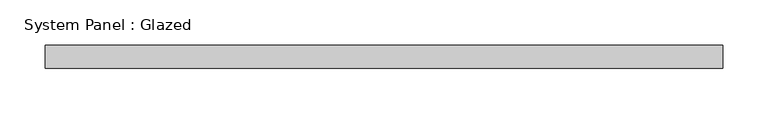
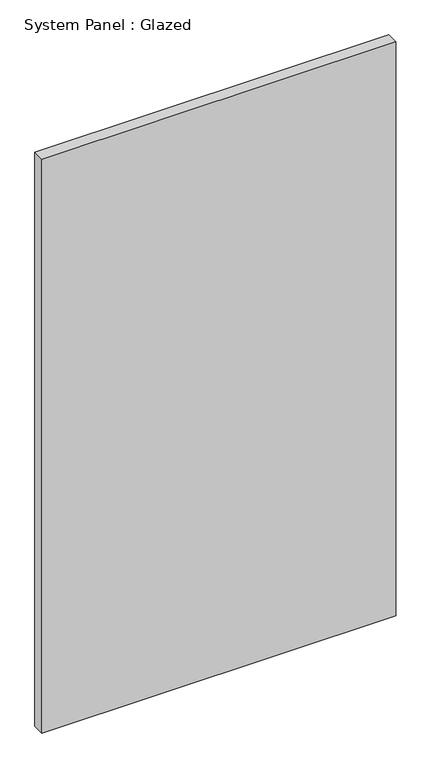
"""IFC4 building model written with IfcOpenShell, lengths in millimetres: plate geometry, System Panel : Glazed."""

from ifc_helpers import new_model, si_unit, origin, origin_with_axes, place, context, project, spatial, polyline, outline, extrude, source, transform, mapped, element, save


def system_panel_glazed_5516fd1f(model_context):
    return source(origin(), model_context, "Body", "SweptSolid", [
        extrude(outline(polyline([(374.65, 19.05), (-374.65, 19.05), (-374.65, 44.45), (374.65, 44.45), (374.65, 19.05)])), origin_with_axes(), (0.0, 0.0, 1.0), 1284.7908292),
    ])


if __name__ == "__main__":
    model = new_model("IFC4")
    model_context = context("Model", 3, world=origin())
    ifc_project = project(units=[si_unit("LENGTHUNIT", "METRE", prefix="MILLI")], contexts=[model_context])
    site = spatial("IfcSite", under=ifc_project)
    building = spatial("IfcBuilding", under=site)
    placement = place(None, origin())
    system_panel_glazed_shape = system_panel_glazed_5516fd1f(model_context)
    element("IfcPlate", 1, ObjectType="System Panel : Glazed", at=placement, inside=building, context=model_context, shape_type="MappedRepresentation", body=[
        mapped(system_panel_glazed_shape, transform((0.0, 0.0, 0.0), x_axis=(1.0, 0.0, 0.0), y_axis=(0.0, 1.0, 0.0), z_axis=(0.0, 0.0, 1.0))),
    ])
    save(model, "model.ifc")

# Revit data of these elements
# Type "System Panel : Glazed"
#   Construction Type Id = "GSP4R"
#   Analytic Construction = "1/8 in Pilkington single glazing"
#   Visual Light Transmittance = 0.9
#   Solar Heat Gain Coefficient = 0.86
#   Heat Transfer Coefficient (U) = 1.18115 BTU/(h·ft²·°F)
#   Define Thermal Properties by = 1
# Element 1 (IfcPlate, "System Panel : Glazed")
#   Materials on its faces: "Glass"
# Materials
#   "Glass": class "Glass", colour RGB 0 128 192, transparency 0.75, Description = "Soda Lime Glass", Cost = 0
